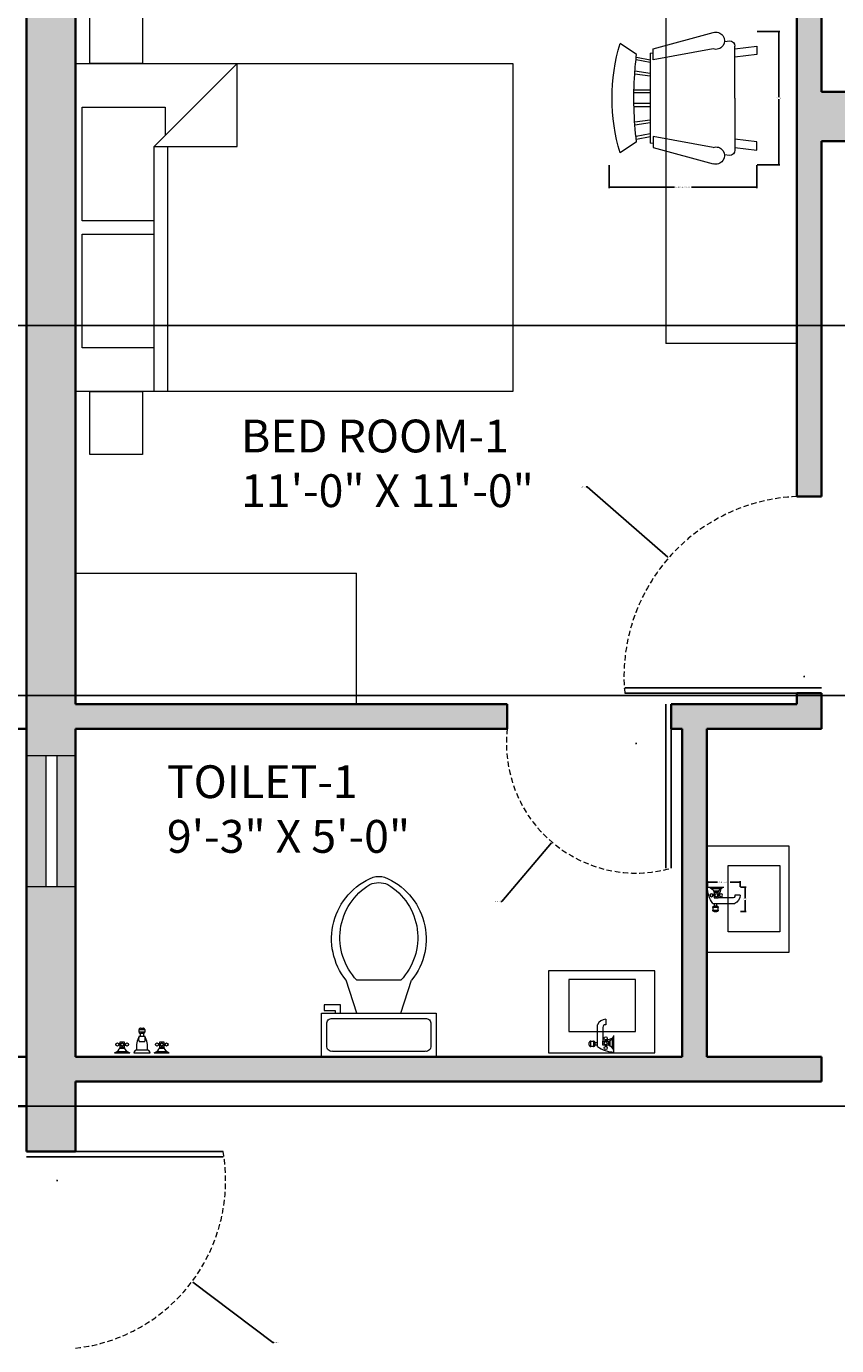
# Model space of a CAD drawing. Units: inches. Extents: x 1693 to 2974, y 2201 to 2965.
# Tile 20 of 24: x 2479 to 2628, y 2588 to 2829. Entities that reach past the tile are written whole.
import ezdxf

# ---------------------------------------------------------------- set-up
doc = ezdxf.new("R2010")
doc.units = ezdxf.units.IN
doc.header["$LTSCALE"] = 2
doc.header["$MEASUREMENT"] = 0
doc.linetypes.add('HIDDEN', pattern=[0.375, 0.25, -0.125])
for name, color, linetype, lineweight in [('A-ANNO-DIMS', 2, 'Continuous', 18), ('A-AREA-IDEN', 7, 'Continuous', 18), ('A-DOOR', 3, 'Continuous', 25), ('A-DOOR-SWNG', 3, 'HIDDEN', 13), ('A-FLOR-CASE', 32, 'Continuous', 18), ('A-FLOR-FIXT', 9, 'Continuous', 18), ('A-FURN', 8, 'Continuous', 18), ('A-GLAZ', 4, 'Continuous', 18), ('A-GLAZ-OVHD', 8, 'HIDDEN', 13), ('A-WALL', 7, 'Continuous', 35)]:
    doc.layers.add(name, color=color, linetype=linetype, lineweight=lineweight)
doc.layers.add('A-GLAZ-PATT', color=141, linetype='Continuous', lineweight=13, true_color=0xadddf7)
doc.layers.add('A-WALL-PATT', color=251, linetype='Continuous', lineweight=13, true_color=0x636466)
doc.styles.get("Standard").update_dxf_attribs({"font": 'arial.ttf'})
doc.dimstyles.get("Standard").update_dxf_attribs({"dimtxt": 0.18, "dimasz": 0.18, "dimexe": 0.18, "dimexo": 0.0625, "dimgap": 0.09, "dimtad": 0, "dimtih": 1, "dimtoh": 1, "dimdec": 1, "dimzin": 0, "dimdsep": 46, "dimlunit": 3, "dimtxsty": 'Standard', "dimcen": 0.09, "dimadec": 0, "dimazin": 0, "dimtfac": 1, "dimtdec": 1, "dimtofl": 0, "dimtmove": 0, "dimatfit": 3, "dimfxl": 1, "dimtolj": 1, "dimtzin": 0, "dimarcsym": 0})

# ---------------------------------------------------------------- blocks, each defined once
blk = doc.blocks.new('Chair - Rocking')
for p, q in [((-8, -4.5), (-10, -1.5)), ((8, -4.5), (10, -1.5)), ((-7.5, -4.5), (-7, -7)), ((-6.5, -7), (-7.02225, -4.43)), ((-4.5, -7), (-4.96674, -4.19951)), ((-4, -7), (-4.40532, -4.16272)), ((-1.5, -4.05012), (-1.5, -7)), ((-1, -7), (-1, -4.05012)), ((1, -7), (1, -4.04655)), ((1.5, -4.05012), (1.5, -7)), ((4, -7), (4.40187, -4.18694)), ((4.5, -7), (4.96761, -4.19437)), ((6.5, -7), (7, -4.4057)), ((7.5, -4.5), (7, -7)), ((-8.23428, -6.99939), (-8.3093, -7.47958)), ((-8.23041, -7), (8.23915, -7)), ((8.31071, -7.48854), (8.23449, -7.00073)), ((-9, -7.5), (-12, -18.49999)), ((-7, -7.5), (-9, -7.5)), ((-9, -18.49999), (-7, -7.5)), ((7, -7.5), (9, -7.5)), ((9, -18.49999), (7, -7.5)), ((9, -7.5), (12, -18.49999)), ((-10.36644, -20.64523), (-10.5, -21.49999)), ((10.5, -21.49999), (10.3575, -20.58798)), ((-9, -22.49999), (-9.5, -26.49999)), ((0, -22.49999), (-9.5, -22.49999)), ((-8, -26.49999), (-7.5, -22.49999)), ((0, -22.49999), (9.5, -22.49999)), ((8, -26.49999), (7.5, -22.49999)), ((9, -22.49999), (9.5, -26.49999)), ((-9.5, -26.49999), (-8, -26.49999)), ((9.5, -26.49999), (8, -26.49999))]:
    blk.add_line(p, q)
for centre, radius, start, end in [((0, -34.08333), 34.08333, 72.93847, 107.0615), ((0, -68.25004), 64.25, 93.92211, 97.15267), ((0, -68.25004), 64.25, 82.84733, 93.92211), ((-10.5, -18.99999), 1.58114, 161.5651, 18.43495), ((10.5, -18.99999), 1.58114, 161.5651, 18.43495), ((-9.5, -21.49999), 1, 180, 270), ((9.5, -21.49999), 1, 270, 0)]:
    blk.add_arc(centre, radius, start, end)
blk = doc.blocks.new('Toilet - top')
for p, q in [((9.5, -6), (9.5, -2)), ((-10, -8.5), (-8, -8.5)), ((-10, -9.5), (-10, -8.5)), ((-7, -9.5), (-10, -9.5)), ((-8, -8.5), (-8, -8)), ((-7, -8), (-7, -9.5)), ((-4, -8), (-6, -14)), ((4, -8), (6, -14)), ((4, -14), (-4, -14))]:
    blk.add_line(p, q)
blk.add_lwpolyline([(10.5, -8), (10.5, 0), (-10.5, 0), (-10.5, -8)], close=True)
for points in [[(-9.5, -2), (-9.5, -6)], [(8.5, -1), (-8.5, -1)], [(-8.5, -7), (8.5, -7)]]:
    blk.add_lwpolyline(points)
for centre, radius, start, end in [((-8.62, -1.88), 0.884, 81.8699, 188.1301), ((8.62, -1.88), 0.884, 351.8699, 98.1301), ((-8.62, -6.12), 0.884, 171.8699, 278.1301), ((8.62, -6.12), 0.884, 261.8699, 8.1301), ((3.52, -21.58), 12.17, 141.4691, 247.9714), ((4.2, -21.82), 11.33, 136.3677, 238.9468), ((-3.52, -21.58), 12.17, 292.0284, 38.5307), ((-4.2, -21.82), 11.33, 301.053, 43.6321), ((0, -27.88), 4, 245.7318, 294.2682), ((0, -29), 4, 254.8605, 285.1395)]:
    blk.add_arc(centre, radius, start, end)
blk = doc.blocks.new('Faucet - Bathroom side')
for p, q in [((-0.625, 4.25), (0.375, 4.25)), ((0.375, 3.75), (-0.625, 3.75)), ((-0.625, 3), (3.375, 3)), ((-0.375, 3), (-0.375, 3.5)), ((0.125, 3.5), (0.125, 3)), ((-1.625, 0), (-1.375, 0)), ((-1.375, 0), (1.375, 0)), ((-0.88366, 0.25), (0.88424, 0.25)), ((-0.375, 1.625), (-0.625, 1.625)), ((-0.375, 1.375), (-0.625, 1.375)), ((0.48078, 0.75), (-0.47286, 0.75)), ((2.875, 2), (0.375, 2)), ((0.375, 1.625), (0.625, 1.625)), ((0.375, 1.375), (0.625, 1.375)), ((4.375, 1.5), (3.375, 1.5))]:
    blk.add_line(p, q)
for points in [[(-0.625, 3.75), (-0.625, 4.25)], [(-0.375, 4.5), (0.125, 4.5)], [(0.125, 3.5), (-0.375, 3.5)], [(0.375, 4.25), (0.375, 3.75)]]:
    blk.add_lwpolyline(points)
blk.add_lwpolyline([(-0.375, 1), (-0.375, 2), (0.375, 2), (0.375, 1)], close=True)
for centre in [(-0.875, 1.5), (0, 1.5), (0.875, 1.5)]:
    blk.add_circle(centre, 0.27951)
for centre, radius, start, end in [((3.45929, -0.0281), 5.08436, 143.4467, 179.6834), ((-0.38253, 4.2575), 0.24259, 88.22243, 181.7776), ((-0.38253, 3.7424), 0.24259, 178.2224, 271.7776), ((0.13252, 4.2575), 0.24259, 358.2224, 91.77757), ((0.13252, 3.7424), 0.24259, 268.2224, 1.777565), ((2.70708, 1.4714), 1.66816, 0.9827695, 66.39737), ((-1.75, 1.375), 1.42522, 285.2551, 344.7449), ((1.75, 1.375), 1.42522, 195.2551, 254.7449), ((-2.49562, -0.286), 3.38273, 9.709485, 29.48735), ((2.96867, 1.5936), 0.41699, 347.0192, 102.9808)]:
    blk.add_arc(centre, radius, start, end)
blk = doc.blocks.new('Faucet - Bathroom front')
for p, q in [((-0.5, 4.25), (0.5, 4.25)), ((0.5, 3.75), (-0.5, 3.75)), ((-0.5, 3), (0.5, 3)), ((-0.25, 3), (-0.25, 3.5)), ((0.25, 3.5), (0.25, 3)), ((-5, 0), (-2.25, 0)), ((-4.5087, 0.25), (-2.7408, 0.25)), ((-4, 1.625), (-4.25, 1.625)), ((-4, 1.375), (-4.25, 1.375)), ((-3.1442, 0.75), (-4.0979, 0.75)), ((-3.25, 1.625), (-3, 1.625)), ((-3.25, 1.375), (-3, 1.375)), ((-1.5, 0), (1.5, 0)), ((-1, 0.5), (1, 0.5)), ((0.5, 2), (-0.5, 2)), ((2.25, 0), (5, 0)), ((2.7413, 0.25), (4.5092, 0.25)), ((3.25, 1.625), (3, 1.625)), ((3.25, 1.375), (3, 1.375)), ((4.1058, 0.75), (3.1521, 0.75)), ((4, 1.625), (4.25, 1.625)), ((4, 1.375), (4.25, 1.375))]:
    blk.add_line(p, q)
for points in [[(-0.5, 3.75), (-0.5, 4.25)], [(-0.25, 4.5), (0.25, 4.5)], [(0.25, 3.5), (-0.25, 3.5)], [(0.5, 4.25), (0.5, 3.75)]]:
    blk.add_lwpolyline(points)
for points in [[(-4, 1), (-4, 2), (-3.25, 2), (-3.25, 1)], [(3.25, 1), (3.25, 2), (4, 2), (4, 1)]]:
    blk.add_lwpolyline(points, close=True)
for centre in [(-4.5, 1.5), (-3.625, 1.5), (-2.75, 1.5), (2.75, 1.5), (3.625, 1.5), (4.5, 1.5)]:
    blk.add_circle(centre, 0.2795)
for centre, radius, start, end in [((3, 1), 4.0311, 150.2551, 187.125), ((0.6413, 2.5), 1.246, 156.3417, 203.6583), ((-0.2575, 4.2575), 0.2426, 88.22243, 181.7776), ((-0.2575, 3.7425), 0.2426, 178.2224, 271.7776), ((0.2575, 4.2575), 0.2426, 358.2224, 91.77757), ((0.2575, 3.7425), 0.2426, 268.2224, 1.777565), ((-3, 1), 4.0311, 352.875, 29.74488), ((-0.6413, 2.5), 1.246, 336.3417, 23.65835), ((-5.375, 1.375), 1.4252, 285.2551, 344.7449), ((-1.875, 1.375), 1.4252, 195.2551, 254.7449), ((-0.7962, -0.2038), 0.7327, 106.1502, 163.8498), ((0.7962, -0.2038), 0.7327, 16.1502, 73.84979), ((1.875, 1.375), 1.4252, 285.2551, 344.7449), ((5.375, 1.375), 1.4252, 195.2551, 254.7449)]:
    blk.add_arc(centre, radius, start, end)
blk = doc.blocks.new('Bed - Queen')
for p, q in [((0, -80.00003), (0, 0)), ((0, 0), (59.99999, 0)), ((59.99999, 0), (59.99999, -80.00003)), ((7.99999, -1.2), (28.79998, -1.2)), ((7.99999, -14.4), (7.99999, -1.2)), ((28.79998, -1.2), (28.79998, -14.4)), ((31.19999, -1.2), (51.99999, -1.2)), ((31.19999, -14.4), (31.19999, -1.2)), ((51.99999, -1.2), (51.99999, -16.4)), ((0, -14.4), (44.8, -14.4)), ((59.99999, -29.6), (44.8, -14.4)), ((44.8, -14.4), (44.8, -29.6)), ((44.8, -16.8), (0, -16.8)), ((51.99999, -16.4), (46.79936, -16.4)), ((44.8, -29.6), (59.99999, -29.6)), ((59.99999, -80.00003), (0, -80.00003))]:
    blk.add_line(p, q)
blk = doc.blocks.new('NIGHTSTAND')
at = {"ltscale": 2}
blk.add_lwpolyline([(11.51, 0), (0, 0), (0, 9.62), (11.51, 9.62)], close=True, dxfattribs=at)
blk = doc.blocks.new('BASIN-WALL-MOUNT')
at = {"ltscale": 2}
for points in [[(15.01, 19.49), (0, 19.49), (0, 0), (15.01, 0)], [(11.1, 15.94), (1.63, 15.94), (1.63, 3.76), (11.1, 3.76)]]:
    blk.add_lwpolyline(points, close=True, dxfattribs=at)
blk = doc.blocks.new('*D33')
at = {"layer": 'A-ANNO-DIMS', "color": 0, "lineweight": -2, "ltscale": 2, "transparency": 16777216}
for p, q in [((2603.86, 2671.88), (2603.86, 2672.9)), ((2604.04, 2672.72), (2605.72, 2672.72)), ((2609.68, 2672.72), (2608.01, 2672.72)), ((2609.86, 2671.88), (2609.86, 2672.9))]:
    blk.add_line(p, q, dxfattribs=at)
at = {"layer": 'A-ANNO-DIMS', "color": 0, "ltscale": 2, "transparency": 16777216}
for points in [[(2604.04, 2672.75), (2604.04, 2672.69), (2603.86, 2672.72)], [(2609.68, 2672.75), (2609.68, 2672.69), (2609.86, 2672.72)]]:
    blk.add_solid(points, dxfattribs=at)
at = {"layer": 'Defpoints', "color": 0, "ltscale": 2, "transparency": 16777216}
for p in [(2603.86, 2671.82), (2609.86, 2672.72), (2609.86, 2671.82)]:
    blk.add_point(p, dxfattribs=at)
at = {"layer": 'A-ANNO-DIMS', "color": 0, "ltscale": 2, "transparency": 16777216, "insert": (2606.86, 2672.72), "char_height": 0.18, "attachment_point": 5}
blk.add_mtext('\\A1;BASIN TAP 6 TYP.', dxfattribs=at)
blk = doc.blocks.new('*D34')
at = {"layer": 'A-ANNO-DIMS', "color": 0, "lineweight": -2, "ltscale": 2, "transparency": 16777216}
for p, q in [((2609.92, 2671.82), (2610.94, 2671.82)), ((2610.76, 2671.64), (2610.76, 2669.75)), ((2610.76, 2667.5), (2610.76, 2669.39)), ((2609.92, 2667.32), (2610.94, 2667.32))]:
    blk.add_line(p, q, dxfattribs=at)
at = {"layer": 'A-ANNO-DIMS', "color": 0, "ltscale": 2, "transparency": 16777216}
for points in [[(2610.73, 2671.64), (2610.79, 2671.64), (2610.76, 2671.82)], [(2610.73, 2667.5), (2610.79, 2667.5), (2610.76, 2667.32)]]:
    blk.add_solid(points, dxfattribs=at)
at = {"layer": 'Defpoints', "color": 0, "ltscale": 2, "transparency": 16777216}
for p in [(2609.86, 2671.82), (2609.86, 2667.32), (2610.76, 2667.32)]:
    blk.add_point(p, dxfattribs=at)
at = {"layer": 'A-ANNO-DIMS', "color": 0, "ltscale": 2, "transparency": 16777216, "insert": (2610.76, 2669.57), "char_height": 0.18, "attachment_point": 5}
blk.add_mtext('\\A1;5 TYP.', dxfattribs=at)
blk = doc.blocks.new('*D39')
at = {"layer": 'A-ANNO-DIMS', "color": 0, "lineweight": -2, "ltscale": 2, "transparency": 16777216}
for p, q in [((2585.91, 2803.84), (2585.91, 2799.68)), ((2612.91, 2803.84), (2612.91, 2799.68)), ((2586.09, 2799.86), (2597.84, 2799.86)), ((2612.73, 2799.86), (2600.98, 2799.86))]:
    blk.add_line(p, q, dxfattribs=at)
at = {"layer": 'A-ANNO-DIMS', "color": 0, "ltscale": 2, "transparency": 16777216}
for points in [[(2586.09, 2799.89), (2586.09, 2799.83), (2585.91, 2799.86)], [(2612.73, 2799.89), (2612.73, 2799.83), (2612.91, 2799.86)]]:
    blk.add_solid(points, dxfattribs=at)
at = {"layer": 'Defpoints', "color": 0, "ltscale": 2, "transparency": 16777216}
for p in [(2585.91, 2803.91), (2612.91, 2803.91), (2585.91, 2799.86)]:
    blk.add_point(p, dxfattribs=at)
at = {"layer": 'A-ANNO-DIMS', "color": 0, "ltscale": 2, "transparency": 16777216, "insert": (2599.41, 2799.86), "char_height": 0.18, "attachment_point": 5}
blk.add_mtext('\\A1;ROCKING CHAIR 27 TYP.', dxfattribs=at)
blk = doc.blocks.new('*D40')
at = {"layer": 'A-ANNO-DIMS', "color": 0, "lineweight": -2, "ltscale": 2, "transparency": 16777216}
for p, q in [((2612.97, 2828.34), (2617.14, 2828.34)), ((2616.96, 2828.16), (2616.96, 2816.3)), ((2616.96, 2804.09), (2616.96, 2815.94)), ((2612.97, 2803.91), (2617.14, 2803.91))]:
    blk.add_line(p, q, dxfattribs=at)
at = {"layer": 'A-ANNO-DIMS', "color": 0, "ltscale": 2, "transparency": 16777216}
for points in [[(2616.93, 2828.16), (2616.99, 2828.16), (2616.96, 2828.34)], [(2616.93, 2804.09), (2616.99, 2804.09), (2616.96, 2803.91)]]:
    blk.add_solid(points, dxfattribs=at)
at = {"layer": 'Defpoints', "color": 0, "ltscale": 2, "transparency": 16777216}
for p in [(2612.91, 2828.34), (2612.91, 2803.91), (2616.96, 2803.91)]:
    blk.add_point(p, dxfattribs=at)
at = {"layer": 'A-ANNO-DIMS', "color": 0, "ltscale": 2, "transparency": 16777216, "insert": (2616.96, 2816.12), "char_height": 0.18, "attachment_point": 5}
blk.add_mtext('\\A1;24 TYP.', dxfattribs=at)
blk = doc.blocks.new('*D81')
at = {"layer": 'A-ANNO-DIMS', "color": 0, "lineweight": -2, "ltscale": 2, "transparency": 16777216}
for p, q in [((1752.34, 2553.91), (1752.34, 2964.96)), ((1752.52, 2964.78), (2332.94, 2964.78)), ((2914.06, 2964.78), (2333.64, 2964.78)), ((2914.24, 2754.97), (2914.24, 2964.96))]:
    blk.add_line(p, q, dxfattribs=at)
at = {"layer": 'A-ANNO-DIMS', "color": 0, "ltscale": 2, "transparency": 16777216}
for points in [[(1752.52, 2964.81), (1752.52, 2964.75), (1752.34, 2964.78)], [(2914.06, 2964.81), (2914.06, 2964.75), (2914.24, 2964.78)]]:
    blk.add_solid(points, dxfattribs=at)
at = {"layer": 'Defpoints', "color": 0, "ltscale": 2, "transparency": 16777216}
for p in [(2914.24, 2964.78), (2914.24, 2754.9), (1752.34, 2553.84)]:
    blk.add_point(p, dxfattribs=at)
at = {"layer": 'A-ANNO-DIMS', "color": 0, "ltscale": 2, "transparency": 16777216, "insert": (2333.29, 2964.78), "char_height": 0.18, "attachment_point": 5}
blk.add_mtext('\\A1;1162', dxfattribs=at)
blk = doc.blocks.new('*D82')
at = {"layer": 'A-ANNO-DIMS', "color": 0, "lineweight": -2, "ltscale": 2, "transparency": 16777216}
for p, q in [((2615.67, 2906.08), (1693.46, 2906.08)), ((1693.64, 2905.9), (1693.64, 2582.94)), ((1693.64, 2259.62), (1693.64, 2582.58)), ((2096.17, 2259.44), (1693.46, 2259.44))]:
    blk.add_line(p, q, dxfattribs=at)
at = {"layer": 'A-ANNO-DIMS', "color": 0, "ltscale": 2, "transparency": 16777216}
for points in [[(1693.61, 2905.9), (1693.67, 2905.9), (1693.64, 2906.08)], [(1693.61, 2259.62), (1693.67, 2259.62), (1693.64, 2259.44)]]:
    blk.add_solid(points, dxfattribs=at)
at = {"layer": 'Defpoints', "color": 0, "ltscale": 2, "transparency": 16777216}
for p in [(1693.64, 2906.08), (2615.74, 2906.08), (2096.24, 2259.44)]:
    blk.add_point(p, dxfattribs=at)
at = {"layer": 'A-ANNO-DIMS', "color": 0, "ltscale": 2, "transparency": 16777216, "insert": (1693.64, 2582.76), "char_height": 0.18, "attachment_point": 5}
blk.add_mtext('\\A1;646.6', dxfattribs=at)
blk = doc.blocks.new('*D90')
at = {"layer": 'A-ANNO-DIMS', "color": 0, "lineweight": -2, "ltscale": 2, "transparency": 16777216}
for p, q in [((2145.8, 2774.54), (2973.12, 2774.54)), ((2972.94, 2774.36), (2972.94, 2740.87)), ((2972.94, 2707.02), (2972.94, 2740.51)), ((2294.3, 2706.84), (2973.12, 2706.84))]:
    blk.add_line(p, q, dxfattribs=at)
at = {"layer": 'A-ANNO-DIMS', "color": 0, "ltscale": 2, "transparency": 16777216}
for points in [[(2972.91, 2774.36), (2972.97, 2774.36), (2972.94, 2774.54)], [(2972.91, 2707.02), (2972.97, 2707.02), (2972.94, 2706.84)]]:
    blk.add_solid(points, dxfattribs=at)
at = {"layer": 'Defpoints', "color": 0, "ltscale": 2, "transparency": 16777216}
for p in [(2145.74, 2774.54), (2294.24, 2706.84), (2972.94, 2706.84)]:
    blk.add_point(p, dxfattribs=at)
at = {"layer": 'A-ANNO-DIMS', "color": 0, "ltscale": 2, "transparency": 16777216, "insert": (2972.94, 2740.69), "char_height": 0.18, "attachment_point": 5}
blk.add_mtext('\\A1;67.7', dxfattribs=at)
blk = doc.blocks.new('*D97')
at = {"layer": 'A-ANNO-DIMS', "color": 0, "lineweight": -2, "ltscale": 2, "transparency": 16777216}
for p, q in [((2294.3, 2631.75), (2973.12, 2631.75)), ((2972.94, 2631.57), (2972.94, 2609.19)), ((2972.94, 2586.44), (2972.94, 2608.83)), ((2294.3, 2586.26), (2973.12, 2586.26))]:
    blk.add_line(p, q, dxfattribs=at)
at = {"layer": 'A-ANNO-DIMS', "color": 0, "ltscale": 2, "transparency": 16777216}
for points in [[(2972.91, 2631.57), (2972.97, 2631.57), (2972.94, 2631.75)], [(2972.91, 2586.44), (2972.97, 2586.44), (2972.94, 2586.26)]]:
    blk.add_solid(points, dxfattribs=at)
at = {"layer": 'Defpoints', "color": 0, "ltscale": 2, "transparency": 16777216}
for p in [(2294.24, 2631.75), (2972.94, 2631.75), (2294.24, 2586.26)]:
    blk.add_point(p, dxfattribs=at)
at = {"layer": 'A-ANNO-DIMS', "color": 0, "ltscale": 2, "transparency": 16777216, "insert": (2972.94, 2609.01), "char_height": 0.18, "attachment_point": 5}
blk.add_mtext('\\A1;45.49', dxfattribs=at)
blk = doc.blocks.new('*D114')
at = {"layer": 'A-ANNO-DIMS', "color": 0, "lineweight": -2, "ltscale": 2, "transparency": 16777216}
for p, q in [((2581.68, 2745.05), (2581.86, 2745.05)), ((2581.86, 2745.05), (2596.62, 2732.14)), ((2621.49, 2710.3), (2621.67, 2710.3)), ((2621.58, 2710.21), (2621.58, 2710.39))]:
    blk.add_line(p, q, dxfattribs=at)
at = {"layer": 'A-ANNO-DIMS', "color": 0, "ltscale": 2, "transparency": 16777216}
blk.add_solid([(2596.64, 2732.16), (2596.6, 2732.11), (2596.76, 2732.02)], dxfattribs=at)
at = {"layer": 'Defpoints', "color": 0, "ltscale": 2, "transparency": 16777216}
for p in [(2596.76, 2732.02), (2621.58, 2710.3)]:
    blk.add_point(p, dxfattribs=at)
at = {"layer": 'A-ANNO-DIMS', "color": 0, "ltscale": 2, "transparency": 16777216, "insert": (2581.13, 2745.05), "char_height": 0.18, "attachment_point": 5}
blk.add_mtext('\\A1;R32.985', dxfattribs=at)
blk = doc.blocks.new('*D118')
at = {"layer": 'A-ANNO-DIMS', "color": 0, "lineweight": -2, "ltscale": 2, "transparency": 16777216}
for p, q in [((2484.76, 2618.12), (2484.94, 2618.12)), ((2484.85, 2618.03), (2484.85, 2618.21)), ((2524.34, 2588.51), (2509.68, 2599.51)), ((2524.52, 2588.51), (2524.34, 2588.51))]:
    blk.add_line(p, q, dxfattribs=at)
at = {"layer": 'A-ANNO-DIMS', "color": 0, "ltscale": 2, "transparency": 16777216}
blk.add_solid([(2509.69, 2599.53), (2509.66, 2599.48), (2509.53, 2599.61)], dxfattribs=at)
at = {"layer": 'Defpoints', "color": 0, "ltscale": 2, "transparency": 16777216}
for p in [(2484.85, 2618.12), (2509.53, 2599.61)]:
    blk.add_point(p, dxfattribs=at)
at = {"layer": 'A-ANNO-DIMS', "color": 0, "ltscale": 2, "transparency": 16777216, "insert": (2525, 2588.51), "char_height": 0.18, "attachment_point": 5}
blk.add_mtext('\\A1;R30.85', dxfattribs=at)
blk = doc.blocks.new('*D127')
at = {"layer": 'A-ANNO-DIMS', "color": 0, "lineweight": -2, "ltscale": 2, "transparency": 16777216}
for p, q in [((2590.72, 2698.09), (2590.9, 2698.09)), ((2590.81, 2698), (2590.81, 2698.18)), ((2566.23, 2669.17), (2575.33, 2679.88)), ((2566.05, 2669.17), (2566.23, 2669.17))]:
    blk.add_line(p, q, dxfattribs=at)
at = {"layer": 'A-ANNO-DIMS', "color": 0, "ltscale": 2, "transparency": 16777216}
blk.add_solid([(2575.31, 2679.9), (2575.35, 2679.86), (2575.45, 2680.02)], dxfattribs=at)
at = {"layer": 'Defpoints', "color": 0, "ltscale": 2, "transparency": 16777216}
for p in [(2590.81, 2698.09), (2575.45, 2680.02)]:
    blk.add_point(p, dxfattribs=at)
at = {"layer": 'A-ANNO-DIMS', "color": 0, "ltscale": 2, "transparency": 16777216, "insert": (2565.5, 2669.17), "char_height": 0.18, "attachment_point": 5}
blk.add_mtext('\\A1;R23.723', dxfattribs=at)

msp = doc.modelspace()

# ---------------------------------------------------------------- hatches: boundary and pattern name
at = {"layer": 'A-GLAZ-PATT', "ltscale": 2}
h = msp.add_hatch(color=256, dxfattribs=at)
h.dxf.hatch_style = 1
h.paths.add_polyline_path([(2656.9702, 2338.2547), (2632.9702, 2338.2547), (2632.9702, 2339.2547), (2608.9702, 2339.2547), (2608.9702, 2334.7547), (2656.9702, 2334.7547)])
h.paths.add_polyline_path([(2656.9702, 2343.7547), (2608.9702, 2343.7547), (2608.9702, 2340.2547), (2632.9702, 2340.2547), (2632.9702, 2339.2547), (2656.9702, 2339.2547)])
h.paths.add_polyline_path([(2775.7544, 2338.2547), (2751.7544, 2338.2547), (2751.7544, 2334.7547), (2775.7544, 2334.7547)])
h.paths.add_polyline_path([(2775.7544, 2343.7547), (2751.7544, 2343.7547), (2751.7544, 2340.2547), (2775.7544, 2340.2547)])
h.paths.add_polyline_path([(2897.7363, 2568.7999), (2893.2363, 2568.7999), (2893.2363, 2520.7999), (2896.7363, 2520.7999), (2896.7363, 2544.7999), (2897.7363, 2544.7999)])
h.paths.add_polyline_path([(2902.2363, 2568.7999), (2898.7363, 2568.7999), (2898.7363, 2544.7999), (2897.7363, 2544.7999), (2897.7363, 2520.7999), (2902.2363, 2520.7999)])
h.paths.add_polyline_path([(2902.2363, 2637.7547), (2898.7363, 2637.7547), (2898.7363, 2613.7547), (2902.2363, 2613.7547)])
h.paths.add_polyline_path([(2896.7363, 2637.7547), (2893.2363, 2637.7547), (2893.2363, 2613.7547), (2896.7363, 2613.7547)])
h.paths.add_polyline_path([(2902.2363, 2748.903), (2899.0477, 2748.903), (2899.0477, 2724.903), (2898.0477, 2724.903), (2898.0477, 2700.903), (2902.2363, 2700.903)])
h.paths.add_polyline_path([(2898.0477, 2748.903), (2893.2363, 2748.903), (2893.2363, 2700.903), (2897.0477, 2700.903), (2897.0477, 2724.903), (2898.0477, 2724.903)])
h.paths.add_polyline_path([(2851.2363, 2846.2547), (2803.2363, 2846.2547), (2803.2363, 2842.7547), (2827.2363, 2842.7547), (2827.2363, 2841.7547), (2851.2363, 2841.7547)])
h.paths.add_polyline_path([(2851.2363, 2840.7547), (2827.2363, 2840.7547), (2827.2363, 2841.7547), (2803.2363, 2841.7547), (2803.2363, 2837.2547), (2851.2363, 2837.2547)])
h.paths.add_polyline_path([(2578.2363, 2846.2547), (2530.2363, 2846.2547), (2530.2363, 2842.7547), (2554.2363, 2842.7547), (2554.2363, 2841.7547), (2578.2363, 2841.7547)])
h.paths.add_polyline_path([(2578.2363, 2840.7547), (2554.2363, 2840.7547), (2554.2363, 2841.7547), (2530.2363, 2841.7547), (2530.2363, 2837.2547), (2578.2363, 2837.2547)])
h.paths.add_polyline_path([(2732.7363, 2812.7547), (2705.1363, 2812.7547), (2705.1363, 2811.7547), (2676.3363, 2811.7547), (2676.3363, 2812.7547), (2648.7363, 2812.7547), (2648.7363, 2808.2547), (2732.7363, 2808.2547)])
h.paths.add_polyline_path([(2732.7363, 2817.2547), (2648.7363, 2817.2547), (2648.7363, 2813.7547), (2676.3363, 2813.7547), (2676.3363, 2812.7547), (2705.1363, 2812.7547), (2705.1363, 2813.7547), (2732.7363, 2813.7547)])
h.paths.add_polyline_path([(2488.2363, 2695.8203), (2484.7878, 2695.8203), (2484.7878, 2671.8203), (2488.2363, 2671.8203)])
h.paths.add_polyline_path([(2482.7878, 2695.8203), (2479.2363, 2695.8203), (2479.2363, 2671.8203), (2482.7878, 2671.8203)])
h.paths.add_polyline_path([(2488.2363, 2572.4371), (2484.7363, 2572.4371), (2484.7363, 2541.4371), (2483.7363, 2541.4371), (2483.7363, 2512.4371), (2488.2363, 2512.4371)])
h.paths.add_polyline_path([(2482.7363, 2541.4371), (2483.7363, 2541.4371), (2483.7363, 2572.4371), (2479.2363, 2572.4371), (2479.2363, 2512.4371), (2482.7363, 2512.4371)])
h.paths.add_polyline_path([(2248.9863, 2706.8449), (2190.9863, 2706.8449), (2190.9863, 2703.3449), (2219.9863, 2703.3449), (2219.9863, 2702.3449), (2248.9863, 2702.3449)])
h.paths.add_polyline_path([(2248.9863, 2701.3449), (2219.9863, 2701.3449), (2219.9863, 2702.3449), (2190.9863, 2702.3449), (2190.9863, 2697.8449), (2248.9863, 2697.8449)])
h.paths.add_polyline_path([(2151.9207, 2293.3449), (2127.9207, 2293.3449), (2127.9207, 2289.8449), (2151.9207, 2289.8449)])
h.paths.add_polyline_path([(2151.9207, 2298.8449), (2127.9207, 2298.8449), (2127.9207, 2295.3449), (2151.9207, 2295.3449)])
h.paths.add_polyline_path([(2084.023, 2293.3449), (2066.023, 2293.3449), (2066.023, 2294.3449), (2048.023, 2294.3449), (2048.023, 2289.8449), (2084.023, 2289.8449)])
h.paths.add_polyline_path([(2084.023, 2298.8449), (2048.023, 2298.8449), (2048.023, 2295.3449), (2066.023, 2295.3449), (2066.023, 2294.3449), (2084.023, 2294.3449)])
h.paths.add_polyline_path([(1966.0781, 2293.3449), (1948.0781, 2293.3449), (1948.0781, 2294.3449), (1930.0781, 2294.3449), (1930.0781, 2289.8449), (1966.0781, 2289.8449)])
h.paths.add_polyline_path([(1966.0781, 2298.8449), (1930.0781, 2298.8449), (1930.0781, 2295.3449), (1948.0781, 2295.3449), (1948.0781, 2294.3449), (1966.0781, 2294.3449)])
h.paths.add_polyline_path([(1787.2363, 2403.1922), (1782.7363, 2403.1922), (1782.7363, 2355.1922), (1786.2363, 2355.1922), (1786.2363, 2379.1922), (1787.2363, 2379.1922)])
h.paths.add_polyline_path([(1791.7363, 2403.1922), (1788.2363, 2403.1922), (1788.2363, 2379.1922), (1787.2363, 2379.1922), (1787.2363, 2355.1922), (1791.7363, 2355.1922)])
h.paths.add_polyline_path([(1786.2363, 2477.5455), (1782.7363, 2477.5455), (1782.7363, 2453.5455), (1786.2363, 2453.5455)])
h.paths.add_polyline_path([(1791.7363, 2477.5455), (1788.2363, 2477.5455), (1788.2363, 2453.5455), (1791.7363, 2453.5455)])
h.paths.add_polyline_path([(1786.2363, 2621.6433), (1782.7363, 2621.6433), (1782.7363, 2585.6433), (1786.2363, 2585.6433)])
h.paths.add_polyline_path([(1791.7363, 2621.6433), (1788.2363, 2621.6433), (1788.2363, 2585.6433), (1791.7363, 2585.6433)])
h.paths.add_polyline_path([(1908.1286, 2706.8449), (1860.1286, 2706.8449), (1860.1286, 2703.3449), (1884.1286, 2703.3449), (1884.1286, 2702.3449), (1908.1286, 2702.3449)])
h.paths.add_polyline_path([(1908.1286, 2701.3449), (1884.1286, 2701.3449), (1884.1286, 2702.3449), (1860.1286, 2702.3449), (1860.1286, 2697.8449), (1908.1286, 2697.8449)])
h.paths.add_polyline_path([(1973.9863, 2706.8449), (1949.9863, 2706.8449), (1949.9863, 2703.3449), (1973.9863, 2703.3449)])
h.paths.add_polyline_path([(1973.9863, 2701.3449), (1949.9863, 2701.3449), (1949.9863, 2697.8449), (1973.9863, 2697.8449)])
h.paths.add_polyline_path([(2112.7363, 2690.3449), (2028.7363, 2690.3449), (2028.7363, 2686.8449), (2056.3363, 2686.8449), (2056.3363, 2685.8449), (2085.1363, 2685.8449), (2085.1363, 2686.8449), (2112.7363, 2686.8449)])
h.paths.add_polyline_path([(2112.7363, 2685.8449), (2085.1363, 2685.8449), (2085.1363, 2684.8449), (2056.3363, 2684.8449), (2056.3363, 2685.8449), (2028.7363, 2685.8449), (2028.7363, 2681.3449), (2112.7363, 2681.3449)])
h.paths.add_polyline_path([(2422.7363, 2640.7547), (2350.7363, 2640.7547), (2350.7363, 2637.2547), (2386.7363, 2637.2547), (2386.7363, 2636.2547), (2422.7363, 2636.2547)])
h.paths.add_polyline_path([(2422.7363, 2635.2547), (2386.7363, 2635.2547), (2386.7363, 2636.2547), (2350.7363, 2636.2547), (2350.7363, 2631.7547), (2422.7363, 2631.7547)])
at = {"layer": 'A-WALL-PATT', "ltscale": 2}
h = msp.add_hatch(color=256, dxfattribs=at)
h.dxf.hatch_style = 1
h.paths.add_polyline_path([(1928.2363, 2733.2161), (1930.9384, 2733.2161), (1930.9384, 2737.2161), (1923.7363, 2737.2161), (1923.7363, 2706.8449), (1908.1286, 2706.8449), (1908.1286, 2697.8449), (1923.7363, 2697.8449), (1923.7363, 2692.8449), (1928.2363, 2692.8449), (1928.2363, 2697.8449), (1949.9863, 2697.8449), (1949.9863, 2706.8449), (1928.2363, 2706.8449)])
h.paths.add_polyline_path([(2004.7363, 2737.2161), (1995.7363, 2737.2161), (1995.7363, 2706.8449), (1985.6374, 2706.8449), (1973.9863, 2706.8449), (1973.9863, 2697.8449), (2000.2363, 2697.8449), (2000.2363, 2686.5348), (2000.3613, 2686.5348), (2000.3613, 2667.0432), (2000.2363, 2601.8449), (1928.2363, 2601.8449), (1928.2363, 2662.8449), (1923.7363, 2662.8449), (1923.7363, 2595.3449), (1928.2363, 2595.3449), (1928.2363, 2597.3449), (2004.7363, 2597.3449), (2004.7363, 2681.3449), (2012.7814, 2681.3449), (2028.7363, 2681.3449), (2028.7363, 2690.3449), (2004.7363, 2690.3449)])
h.paths.add_polyline_path([(2190.9863, 2706.8449), (2184.9863, 2706.8449), (2145.7363, 2706.8449), (2145.7363, 2765.3449), (2145.7363, 2774.5394), (2136.7363, 2774.5394), (2136.7363, 2756.3449), (2136.7363, 2690.3449), (2112.7363, 2690.3449), (2112.7363, 2681.3449), (2136.7363, 2681.3449), (2136.7363, 2597.3449), (2141.2363, 2597.3449), (2141.2363, 2697.8449), (2190.9863, 2697.8449)])
h.paths.add_polyline_path([(1860.1286, 2706.8449), (1782.7363, 2706.8449), (1782.7363, 2621.6433), (1791.7363, 2621.6433), (1791.7363, 2697.8449), (1860.1286, 2697.8449)])
h.paths.add_polyline_path([(1791.7363, 2585.6433), (1782.7363, 2585.6433), (1782.7363, 2562.8449), (1782.7363, 2553.8449), (1752.3363, 2553.8449), (1752.3363, 2544.2586), (1756.3363, 2544.2586), (1756.3363, 2549.3449), (1782.7363, 2549.3449), (1782.7363, 2489.2404), (1782.7363, 2477.5455), (1791.7363, 2477.5455), (1791.7363, 2493.5991), (1791.6113, 2493.5991), (1791.6113, 2513.0907), (1791.6824, 2533.7198, -0.94742783), (1791.7363, 2534.7168), (1791.7363, 2549.3449), (1863.7363, 2549.3449), (1863.7363, 2513.3449), (1866.7363, 2513.3449), (1866.7363, 2549.3449), (1924.7363, 2549.3449), (1924.7363, 2447.3449), (1924.7363, 2442.8449), (1933.7363, 2442.8449), (1933.7363, 2447.3449), (1928.2363, 2447.3449), (1928.2363, 2559.3449), (1923.7363, 2559.3449), (1923.7363, 2553.8449), (1791.7363, 2553.8449), (1791.7363, 2562.8449)])
h.paths.add_polyline_path([(1791.7363, 2442.8449), (1866.7363, 2442.8449), (1866.7363, 2447.3449), (1866.7363, 2483.3449), (1863.7363, 2483.3449), (1863.7363, 2447.3449), (1791.7363, 2447.3449), (1791.7363, 2453.5455), (1782.7363, 2453.5455), (1782.7363, 2447.3449), (1756.3363, 2447.3449), (1756.3363, 2455.7126), (1752.3363, 2455.7126), (1752.3363, 2442.8449), (1782.7363, 2442.8449), (1782.7363, 2403.1922), (1791.7363, 2403.1922)])
h.paths.add_polyline_path([(1930.0781, 2298.8449), (1791.7363, 2298.8449), (1791.7363, 2355.1922), (1782.7363, 2355.1922), (1782.7363, 2289.8449), (1930.0781, 2289.8449)])
h.paths.add_polyline_path([(2624.7363, 2883.2547), (2624.7363, 2902.6165), (2624.7363, 2906.0761), (2615.7363, 2906.0761), (2615.7363, 2892.2547), (2615.7363, 2846.2547), (2578.2363, 2846.2547), (2578.2363, 2837.2547), (2620.2363, 2837.2547), (2620.2363, 2743.2547), (2624.7363, 2743.2547), (2624.7363, 2808.2547), (2648.7363, 2808.2547), (2648.7363, 2817.2547), (2624.7363, 2817.2547)])
h.paths.add_polyline_path([(2530.2363, 2846.2547), (2479.2363, 2846.2547), (2479.2363, 2695.8203), (2488.2363, 2695.8203), (2488.2363, 2700.7547), (2567.2363, 2700.7547), (2567.2363, 2705.2547), (2488.2363, 2705.2547), (2488.2363, 2837.2547), (2530.2363, 2837.2547)])
h.paths.add_polyline_path([(2488.2363, 2487.7547), (2630.2363, 2487.7547, -0.00990191), (2630.2363, 2489.0322), (2630.2363, 2492.2547), (2488.2363, 2492.2547), (2488.2363, 2512.4371), (2479.2363, 2512.4371), (2479.2363, 2334.7547), (2608.9702, 2334.7547), (2608.9702, 2343.7547), (2488.2363, 2343.7547)])
h.paths.add_polyline_path([(2751.7544, 2343.7547), (2672.7363, 2343.7547), (2672.7363, 2409.7547), (2674.7363, 2409.7547), (2674.7363, 2413.7547), (2672.7363, 2413.7547), (2672.7363, 2487.7547), (2732.7363, 2487.7547), (2732.7363, 2413.7547), (2704.7363, 2413.7547), (2704.7363, 2409.7547), (2784.7363, 2409.7547), (2784.7363, 2343.7547), (2775.7544, 2343.7547), (2775.7544, 2334.7547), (2902.2363, 2334.7547), (2902.2363, 2520.7999), (2893.2363, 2520.7999), (2893.2363, 2413.7547), (2856.0145, 2413.7547), (2856.0145, 2409.7547), (2893.2363, 2409.7547), (2893.2363, 2343.7547), (2789.2363, 2343.7547), (2789.2363, 2409.7547), (2819.2363, 2409.7547), (2826.0145, 2409.7547), (2826.0145, 2413.7547), (2789.2363, 2413.7547), (2789.2363, 2492.2547), (2784.7363, 2492.2547), (2784.7363, 2413.7547), (2736.7363, 2413.7547), (2736.7363, 2492.2547), (2672.7363, 2492.2547), (2666.2363, 2492.2547), (2666.2363, 2487.7547), (2668.2363, 2487.7547), (2668.2363, 2343.7547), (2656.9702, 2343.7547), (2656.9702, 2334.7547), (2662.9702, 2334.7547), (2751.7544, 2334.7547)])
h.paths.add_polyline_path([(2902.2363, 2613.7547), (2893.2363, 2613.7547), (2893.2363, 2589.7547), (2785.2363, 2589.7547), (2785.2363, 2661.7547), (2790.2363, 2661.7547), (2790.2363, 2665.2547), (2761.2363, 2665.2547), (2761.2363, 2667.2547), (2756.7363, 2667.2547), (2756.7363, 2661.7547), (2781.2363, 2661.7547), (2781.2363, 2585.7547), (2893.2363, 2585.7547), (2893.2363, 2568.7999), (2902.2363, 2568.7999)])
h.paths.add_polyline_path([(2488.2363, 2671.8203), (2479.2363, 2671.8203), (2479.2363, 2645.2547), (2479.2363, 2623.4598), (2488.2363, 2623.4598), (2488.2363, 2636.2547), (2624.7363, 2636.2547), (2624.7363, 2640.7547), (2603.7363, 2640.7547), (2603.7363, 2700.7547), (2624.7363, 2700.7547), (2624.7363, 2707.2547), (2620.2363, 2707.2547), (2620.2363, 2705.2547), (2597.2363, 2705.2547), (2597.2363, 2700.7547), (2599.2363, 2700.7547), (2599.2363, 2640.7547), (2488.2363, 2640.7547)])
h.paths.add_polyline_path([(2761.2363, 2837.2547), (2803.2363, 2837.2547), (2803.2363, 2846.2547), (2797.2363, 2846.2547), (2765.7363, 2846.2547), (2756.7363, 2846.2547), (2756.7363, 2817.2547), (2732.7363, 2817.2547), (2732.7363, 2808.2547), (2756.7363, 2808.2547), (2756.7363, 2703.2547), (2761.2363, 2703.2547)])
h.paths.add_polyline_path([(2739.7489, 2433.1234), (2786.9181, 2433.1234), (2786.9181, 2455.5122), (2739.7489, 2455.5122)], flags=25)

# ---------------------------------------------------------------- linework, layer by layer
at = {"layer": 'A-DOOR', "ltscale": 2}
for p, q in [((2624.7363, 2708.2547), (2588.7363, 2708.2547)), ((2624.7363, 2707.2547), (2588.7363, 2707.2547)), ((2596.2363, 2705.2547), (2596.2363, 2675.2547)), ((2597.2363, 2705.2547), (2597.2363, 2675.2547)), ((2479.2363, 2623.4598), (2515.2363, 2623.4598)), ((2479.2363, 2622.4598), (2515.2363, 2622.4598))]:
    msp.add_line(p, q, dxfattribs=at)
at = {"layer": 'A-DOOR-SWNG', "ltscale": 2}
for centre, radius, start, end in [((2621.5806, 2710.2972), 32.9849, 92.335719, 185.292431), ((2590.8097, 2698.0911), 23.7234, 173.553414, 285.717513), ((2484.8526, 2618.1226), 30.8489, 276.297258, 9.962947)]:
    msp.add_arc(centre, radius, start, end, dxfattribs=at)
at = {"layer": 'A-FLOR-CASE'}
msp.add_line((2596.2363, 2837.2547), (2596.2363, 2771.2547), dxfattribs=at)
at = {"layer": 'A-FLOR-CASE', "ltscale": 2}
for p, q in [((2620.2363, 2771.2547), (2596.2363, 2771.2547)), ((2488.2363, 2729.2547), (2539.6739, 2729.2547)), ((2539.6739, 2705.2547), (2539.6739, 2729.2547))]:
    msp.add_line(p, q, dxfattribs=at)
at = {"layer": 'A-GLAZ', "ltscale": 2}
for p, q in [((2488.3392, 2695.8203), (2479.2363, 2695.8203)), ((2482.7878, 2695.8203), (2482.7878, 2671.8203)), ((2484.7878, 2695.8203), (2484.7878, 2671.8203)), ((2488.3392, 2671.8203), (2479.2363, 2671.8203))]:
    msp.add_line(p, q, dxfattribs=at)
at = {"layer": 'A-GLAZ-OVHD', "ltscale": 2}
msp.add_line((2479.2363, 2761.3526), (2479.2363, 2767.3526), dxfattribs=at)
at = {"layer": 'A-WALL'}
for p, q in [((2624.7363, 2883.2547), (2624.7363, 2817.2547)), ((2479.2363, 2846.2547), (2479.2363, 2645.2547)), ((2488.2363, 2837.2547), (2488.2363, 2705.2547)), ((2620.2363, 2837.2547), (2620.2363, 2743.2547)), ((2624.7363, 2808.2547), (2624.7363, 2743.2547)), ((2620.2363, 2707.2547), (2620.2363, 2705.2547)), ((2624.7363, 2707.2547), (2624.7363, 2700.7547)), ((2488.2363, 2700.7547), (2488.2363, 2640.7547)), ((2599.2363, 2700.7547), (2599.2363, 2640.7547)), ((2603.7363, 2700.7547), (2603.7363, 2640.7547)), ((2479.2363, 2646.5548), (2479.2363, 2623.4598)), ((2488.2363, 2636.2547), (2488.2363, 2623.4598))]:
    msp.add_line(p, q, dxfattribs=at)
at = {"layer": 'A-WALL', "ltscale": 2}
for p, q in [((2624.7363, 2817.2547), (2756.7363, 2817.2547)), ((2624.7363, 2808.2547), (2756.7363, 2808.2547)), ((2620.2363, 2743.2547), (2624.7363, 2743.2547)), ((2620.2363, 2707.2547), (2624.7363, 2707.2547)), ((2488.2363, 2705.2547), (2567.2363, 2705.2547)), ((2567.2363, 2700.7547), (2567.2363, 2705.2547)), ((2597.2363, 2700.7547), (2597.2363, 2705.2547)), ((2597.2363, 2705.2547), (2620.2363, 2705.2547)), ((2294.166, 2700.7547), (2479.2363, 2700.7547)), ((2488.2363, 2700.7547), (2567.2363, 2700.7547)), ((2597.2363, 2700.7547), (2599.2363, 2700.7547)), ((2603.7363, 2700.7547), (2624.7363, 2700.7547)), ((2479.2363, 2640.7547), (2294.2363, 2640.7547)), ((2488.2363, 2640.7547), (2599.2363, 2640.7547)), ((2603.7363, 2640.7547), (2624.7363, 2640.7547)), ((2624.7363, 2640.7547), (2624.7363, 2636.2547)), ((2488.2363, 2636.2547), (2624.7363, 2636.2547)), ((2479.2363, 2631.7547), (2294.2363, 2631.7547)), ((2479.2363, 2623.4598), (2488.2363, 2623.4598))]:
    msp.add_line(p, q, dxfattribs=at)

# ---------------------------------------------------------------- block references
at = {"layer": 'A-FLOR-FIXT', "extrusion": (0, 0, -1), "zscale": -1}
msp.add_blockref('BASIN-WALL-MOUNT', (-2618.7496, 2659.8373), dxfattribs=at)
at = {"layer": 'A-FLOR-FIXT', "ltscale": 2, "xscale": -1, "rotation": 180}
for name, p in [('Toilet - top', (2543.7363, 2640.7547)), ('Faucet - Bathroom side', (2605.4863, 2671.8181))]:
    msp.add_blockref(name, p, dxfattribs=at)
at = {"layer": 'A-FLOR-FIXT', "rotation": 270.0000000000015}
msp.add_blockref('BASIN-WALL-MOUNT', (2574.7747, 2656.5136), dxfattribs=at)
at = {"layer": 'A-FLOR-FIXT', "ltscale": 2, "rotation": 89.99999999999996}
msp.add_blockref('Faucet - Bathroom side', (2586.7556, 2643.2503), dxfattribs=at)
at = {"layer": 'A-FLOR-FIXT', "ltscale": 2}
msp.add_blockref('Faucet - Bathroom front', (2500.3898, 2641.5067), dxfattribs=at)
at = {"layer": 'A-FURN'}
for p, rotation in [((2490.8504, 2833.9797), 270.0000000000035), ((2490.8504, 2762.4699), 270.0000000000017)]:
    msp.add_blockref('NIGHTSTAND', p, dxfattribs=dict(at, rotation=rotation))
at = {"layer": 'A-FURN', "ltscale": 2, "xscale": -1, "rotation": 90}
msp.add_blockref('Chair - Rocking', (2586.4074, 2816.124), dxfattribs=at)
at = {"layer": 'A-FURN', "ltscale": 2, "rotation": 89.99999999999999}
msp.add_blockref('Bed - Queen', (2488.2363, 2762.4698), dxfattribs=at)

# ---------------------------------------------------------------- texts
at = {"layer": 'A-AREA-IDEN', "ltscale": 2, "char_height": 6, "attachment_point": 1}
for s, insert in [('BED ROOM-1\\P11\'-0" X 11\'-0"', (2518.5074, 2757.3192)), ('TOILET-1\\P9\'-3" X 5\'-0"', (2504.9422, 2694.0798))]:
    msp.add_mtext_dynamic_manual_height_columns(s, width=108.452746, gutter_width=1, heights=[0], dxfattribs=dict(at, insert=insert))

# ---------------------------------------------------------------- dimensions: what is measured, and where the dimension line sits
at = {"layer": 'A-ANNO-DIMS', "ltscale": 2}
dim = msp.add_linear_dim(base=(2914.2363, 2964.7761), p1=(1752.3363, 2553.8449), p2=(2914.2363, 2754.903), dimstyle='Standard', override={"dimdec": 0, "dimlfac": 1, "dimrnd": 0, "dimzin": 0, "dimdsep": 46, "dimlunit": 2}, dxfattribs=at)
dim.commit()
dim.dimension.update_dxf_attribs({"geometry": '*D81', "text_midpoint": (2333.2863, 2964.7761)})
for base, p1, p2, override, picture, middle in [((1693.6363, 2906.0761), (2096.2363, 2259.4449), (2615.7363, 2906.0761), {"dimdec": 1, "dimlfac": 1, "dimrnd": 0, "dimzin": 0, "dimdsep": 46, "dimlunit": 2}, '*D82', (1693.6363, 2582.7605)), ((2972.9363, 2706.8449), (2145.7363, 2774.5394), (2294.2363, 2706.8449), {"dimdec": 1, "dimlfac": 1, "dimrnd": 0, "dimzin": 0, "dimdsep": 46, "dimlunit": 2}, '*D90', (2972.9363, 2740.6922)), ((2972.9363, 2631.7547), (2294.2363, 2586.2648), (2294.2363, 2631.7547), {"dimdec": 2, "dimlfac": 1, "dimrnd": 0, "dimzin": 0, "dimdsep": 46, "dimlunit": 2}, '*D97', (2972.9363, 2609.0097))]:
    dim = msp.add_linear_dim(base=base, p1=p1, p2=p2, angle=90, dimstyle='Standard', override=override, dxfattribs=at)
    dim.commit()
    dim.dimension.update_dxf_attribs({"geometry": picture, "text_midpoint": middle})
for base, p1, p2, angle, text, picture, middle in [((2616.9574, 2803.9065), (2612.9074, 2828.3416), (2612.9074, 2803.9065), 270, '<> TYP.', '*D40', (2616.9574, 2816.124)), ((2585.9074, 2799.8565), (2612.9074, 2803.9065), (2585.9074, 2803.9065), 180, 'ROCKING CHAIR <> TYP.', '*D39', (2599.4074, 2799.8565)), ((2610.7613, 2667.3161), (2609.8613, 2671.8181), (2609.8613, 2667.3161), 270, '<> TYP.', '*D34', (2610.7613, 2669.5671))]:
    dim = msp.add_linear_dim(base=base, p1=p1, p2=p2, angle=angle, text=text, dimstyle='Standard', override={"dimdec": 0, "dimlfac": 1, "dimrnd": 0, "dimzin": 0, "dimdsep": 46, "dimlunit": 2}, dxfattribs=at)
    dim.commit()
    dim.dimension.update_dxf_attribs({"geometry": picture, "text_midpoint": middle})
for center, mpoint, override, picture, middle in [((2621.5806, 2710.2972), (2596.757, 2732.018), {"dimdec": 3, "dimlfac": 1, "dimrnd": 0, "dimzin": 0, "dimdsep": 46, "dimlunit": 2}, '*D114', (2581.1324, 2745.0505)), ((2590.8097, 2698.0911), (2575.4453, 2680.0153), {"dimdec": 3, "dimlfac": 1, "dimrnd": 0, "dimzin": 0, "dimdsep": 46, "dimlunit": 2}, '*D127', (2565.4968, 2669.1698)), ((2484.8526, 2618.1226), (2509.5317, 2599.6132), {"dimdec": 2, "dimlfac": 1, "dimrnd": 0, "dimzin": 0, "dimdsep": 46, "dimlunit": 2}, '*D118', (2524.9997, 2588.5076))]:
    dim = msp.add_radius_dim(center=center, mpoint=mpoint, dimstyle='Standard', override=override, dxfattribs=at)
    dim.commit()
    dim.dimension.update_dxf_attribs({"geometry": picture, "text_midpoint": middle, "dimtype": 164})
dim = msp.add_linear_dim(base=(2609.8613, 2672.7181), p1=(2603.8613, 2671.8181), p2=(2609.8613, 2671.8181), text='BASIN TAP <> TYP.', dimstyle='Standard', override={"dimdec": 0, "dimlfac": 1, "dimrnd": 0, "dimzin": 0, "dimdsep": 46, "dimlunit": 2}, dxfattribs=at)
dim.commit()
dim.dimension.update_dxf_attribs({"geometry": '*D33', "text_midpoint": (2606.8613, 2672.7181)})

doc.saveas('drawing.dxf')
